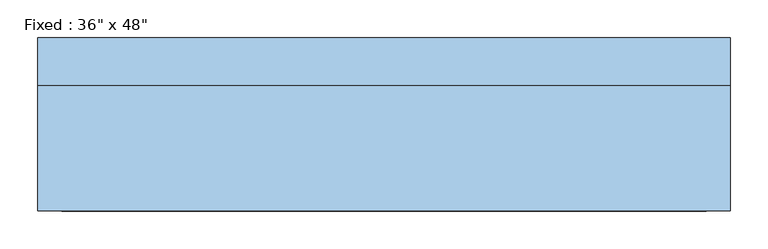
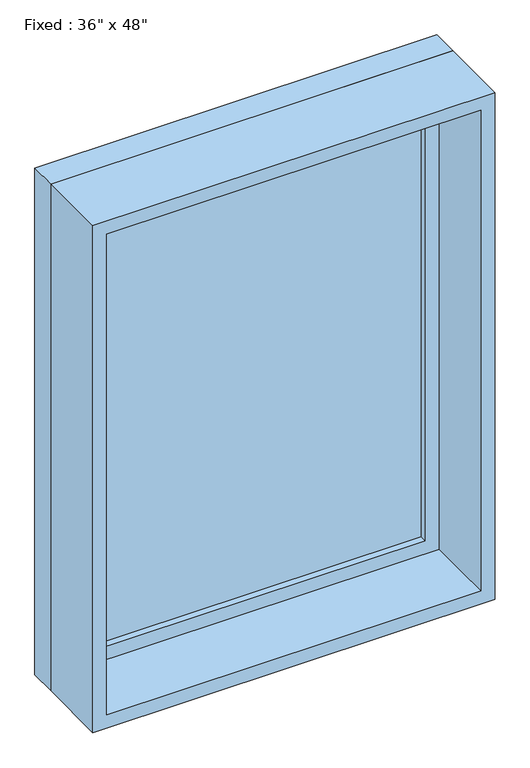
"""IFC4 building model written with IfcOpenShell, lengths in millimetres: window geometry."""

from ifc_helpers import new_model, si_unit, frame, origin, place, context, project, spatial, polyline, outline, extrude, source, transform, mapped, element, save


def window_c1f32544(model_context):
    return source(origin(), model_context, "Body", "SweptSolid", [
        extrude(outline(polyline([(355.6, 66.675), (-431.8, 66.675), (-431.8, 79.375), (355.6, 79.375), (355.6, 66.675)])), frame((0.0, 0.0, 977.9), z_axis=(0.0, 0.0, 1.0), x_axis=(1.0, 0.0, 0.0)), (0.0, 0.0, 1.0), 1092.2),
        extrude(outline(polyline([(2114.55, -476.25), (933.45, -476.25), (933.45, 400.05), (2114.55, 400.05), (2114.55, -476.25)]), holes=[polyline([(2070.1, -431.8), (2070.1, 355.6), (977.9, 355.6), (977.9, -431.8), (2070.1, -431.8)])]), frame((0.0, 50.8, 0.0), z_axis=(0.0, 1.0, 0.0), x_axis=(0.0, 0.0, 1.0)), (0.0, 0.0, 1.0), 44.45),
        extrude(outline(polyline([(2133.6, -495.3), (914.4, -495.3), (914.4, 419.1), (2133.6, 419.1), (2133.6, -495.3)]), holes=[polyline([(2101.85, -463.55), (2101.85, 387.35), (946.15, 387.35), (946.15, -463.55), (2101.85, -463.55)])]), frame((0.0, -114.3, 0.0), z_axis=(0.0, 1.0, 0.0), x_axis=(0.0, 0.0, 1.0)), (0.0, 0.0, 1.0), 165.1),
        extrude(outline(polyline([(2133.6, 419.1), (2133.6, -495.3), (914.4, -495.3), (914.4, 419.1), (2133.6, 419.1)]), holes=[polyline([(2114.55, 400.05), (933.45, 400.05), (933.45, -476.25), (2114.55, -476.25), (2114.55, 400.05)])]), frame((0.0, 50.8, 0.0), z_axis=(0.0, 1.0, 0.0), x_axis=(0.0, 0.0, 1.0)), (0.0, 0.0, 1.0), 63.5),
    ])


if __name__ == "__main__":
    model = new_model("IFC4")
    model_context = context("Model", 3, world=origin())
    ifc_project = project(units=[si_unit("LENGTHUNIT", "METRE", prefix="MILLI")], contexts=[model_context])
    site = spatial("IfcSite", under=ifc_project)
    building = spatial("IfcBuilding", under=site)
    placement = place(None, origin())
    window_shape = window_c1f32544(model_context)
    element("IfcWindow", 1, ObjectType="Fixed : 36\" x 48\"", at=placement, inside=building, context=model_context, shape_type="MappedRepresentation", body=[
        mapped(window_shape, transform((0.0, 0.0, 0.0), x_axis=(1.0, 0.0, 0.0), y_axis=(0.0, 1.0, 0.0), z_axis=(0.0, 0.0, 1.0))),
    ])
    save(model, "model.ifc")

# Revit data of these elements
# Type "Fixed : 36\" x 48\""
#   Type Mark = "W1"
#   Construction Type Id = "GSP4R"
#   Assembly Code = "B2020100"
#   Analytic Construction = "1/8 in Pilkington single glazing"
#   Visual Light Transmittance = 0.9
#   Solar Heat Gain Coefficient = 0.78
#   Heat Transfer Coefficient (U) = 0.6496 BTU/(h·ft²·°F)
#   Height = 4' - 0"
#   Default Sill Height = 3' - 0"
#   Width = 3' - 0"
#   Window Inset = 0' - 0 3/4"
#   Define Thermal Properties by = 1
#   Define Thermal Properties by = 1
#   Glass Pane Material = Glass
#   Sash Material = Sash
#   Wall Closure = (empty or 0)
# Element 1 (IfcWindow, "Fixed : 36\" x 48\"")
#   Materials on its faces: "Sash", "Glass"
# Materials
#   "Glass": class "Glass", colour RGB 0 128 192, transparency 0.75, Description = "Soda Lime Glass", Cost = 0
#   "Sash": class "Wood", colour RGB 224 178 126, transparency 0, Cost = 0
